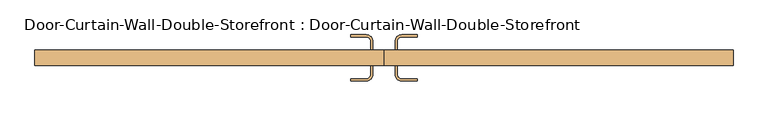
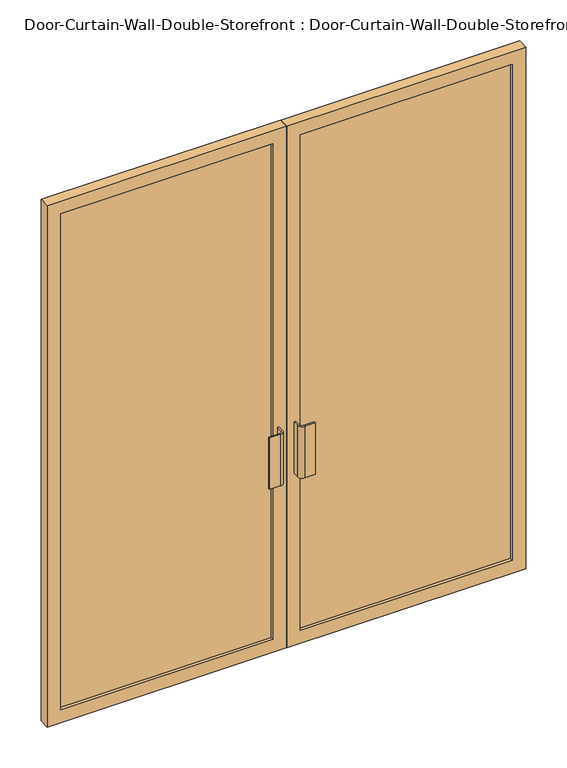
"""IFC4 building model written with IfcOpenShell, lengths in millimetres: door geometry, Door-Curtain-Wall-Double-Storefront : Door-Curtain-Wall-Double-Storefront."""

from ifc_helpers import new_model, si_unit, point, frame, frame_2d, origin, place, context, project, spatial, polyline, circle_curve, trimmed, segment, composite_curve, outline, extrude, source, transform, mapped, element, save


def door_curtain_wall_double_storefront_door_curtain_wall_double_726648f4(model_context):
    return source(origin(), model_context, "Body", "SweptSolid", [
        extrude(outline(polyline([(2311.4, 0.7668501), (0.0, 0.7668501), (0.0, 1003.3), (2311.4, 1003.3), (2311.4, 0.7668501)]), holes=[polyline([(2254.25, 57.9168501), (2254.25, 946.15), (57.15, 946.15), (57.15, 57.9168501), (2254.25, 57.9168501)])]), frame((0.0, 12.7, 0.0), z_axis=(0.0, 1.0, 0.0), x_axis=(0.0, 0.0, 1.0)), (0.0, 0.0, 1.0), 44.45),
        extrude(outline(polyline([(2311.4, -0.8206499), (2311.4, -1003.3), (0.0, -1003.3), (0.0, -0.8206499), (2311.4, -0.8206499)]), holes=[polyline([(2254.25, -946.15), (2254.25, -57.9706499), (57.15, -57.9706499), (57.15, -946.15), (2254.25, -946.15)])]), frame((0.0, 12.7, 0.0), z_axis=(0.0, 1.0, 0.0), x_axis=(0.0, 0.0, 1.0)), (0.0, 0.0, 1.0), 44.45),
        extrude(outline(polyline([(946.15, 25.4), (57.9168501, 25.4), (57.9168501, 44.45), (946.15, 44.45), (946.15, 25.4)])), frame((0.0, 0.0, 57.15), z_axis=(0.0, 0.0, 1.0), x_axis=(1.0, 0.0, 0.0)), (0.0, 0.0, 1.0), 2197.1),
        extrude(outline(polyline([(-57.9706499, 25.4), (-946.15, 25.4), (-946.15, 44.45), (-57.9706499, 44.45), (-57.9706499, 25.4)])), frame((0.0, 0.0, 57.15), z_axis=(0.0, 0.0, 1.0), x_axis=(1.0, 0.0, 0.0)), (0.0, 0.0, 1.0), 2197.1),
        extrude(outline(composite_curve([segment(polyline([(-31.7768999, 82.55), (-31.7768999, 57.15), (-38.1268999, 57.15), (-38.1268999, 82.55)]), True, "CONTINUOUS"), segment(trimmed(circle_curve(frame_2d((-50.8268999, 82.55)), 12.7), [point((-38.1268999, 82.55))], [point((-50.8268999, 95.25))], True, "CARTESIAN"), True, "CONTINUOUS"), segment(polyline([(-50.8268999, 95.25), (-95.2768999, 95.25), (-95.2768999, 101.6), (-50.8268999, 101.6)]), True, "CONTINUOUS"), segment(trimmed(circle_curve(frame_2d((-50.8268999, 82.55)), 19.05), [point((-50.8268999, 101.6))], [point((-31.7768999, 82.55))], False, "CARTESIAN"), True, "CONTINUOUS")], self_intersect=False)), frame((0.0, 0.0, 762.0), z_axis=(0.0, 0.0, 1.0), x_axis=(1.0, 0.0, 0.0)), (0.0, 0.0, 1.0), 228.6),
        extrude(outline(composite_curve([segment(trimmed(circle_curve(frame_2d((50.7731001, 82.55)), 19.05), [point((31.7231001, 82.55))], [point((50.7731001, 101.6))], False, "CARTESIAN"), True, "CONTINUOUS"), segment(polyline([(50.7731001, 101.6), (95.2231001, 101.6), (95.2231001, 95.25), (50.7731001, 95.25)]), True, "CONTINUOUS"), segment(trimmed(circle_curve(frame_2d((50.7731001, 82.55)), 12.7), [point((50.7731001, 95.25))], [point((38.0731001, 82.55))], True, "CARTESIAN"), True, "CONTINUOUS"), segment(polyline([(38.0731001, 82.55), (38.0731001, 57.15), (31.7231001, 57.15), (31.7231001, 82.55)]), True, "CONTINUOUS")], self_intersect=False)), frame((0.0, 0.0, 762.0), z_axis=(0.0, 0.0, 1.0), x_axis=(1.0, 0.0, 0.0)), (0.0, 0.0, 1.0), 228.6),
        extrude(outline(composite_curve([segment(trimmed(circle_curve(frame_2d((-50.8268999, -12.7)), 19.05), [point((-31.7768999, -12.7))], [point((-50.8268999, -31.75))], False, "CARTESIAN"), True, "CONTINUOUS"), segment(polyline([(-50.8268999, -31.75), (-95.2768999, -31.75), (-95.2768999, -25.4), (-50.8268999, -25.4)]), True, "CONTINUOUS"), segment(trimmed(circle_curve(frame_2d((-50.8268999, -12.7)), 12.7), [point((-50.8268999, -25.4))], [point((-38.1268999, -12.7))], True, "CARTESIAN"), True, "CONTINUOUS"), segment(polyline([(-38.1268999, -12.7), (-38.1268999, 12.7), (-31.7768999, 12.7), (-31.7768999, -12.7)]), True, "CONTINUOUS")], self_intersect=False)), frame((0.0, 0.0, 762.0), z_axis=(0.0, 0.0, 1.0), x_axis=(1.0, 0.0, 0.0)), (0.0, 0.0, 1.0), 228.6),
        extrude(outline(composite_curve([segment(polyline([(31.7231001, -12.7), (31.7231001, 12.7), (38.0731001, 12.7), (38.0731001, -12.7)]), True, "CONTINUOUS"), segment(trimmed(circle_curve(frame_2d((50.7731001, -12.7)), 12.7), [point((38.0731001, -12.7))], [point((50.7731001, -25.4))], True, "CARTESIAN"), True, "CONTINUOUS"), segment(polyline([(50.7731001, -25.4), (95.2231001, -25.4), (95.2231001, -31.75), (50.7731001, -31.75)]), True, "CONTINUOUS"), segment(trimmed(circle_curve(frame_2d((50.7731001, -12.7)), 19.05), [point((50.7731001, -31.75))], [point((31.7231001, -12.7))], False, "CARTESIAN"), True, "CONTINUOUS")], self_intersect=False)), frame((0.0, 0.0, 762.0), z_axis=(0.0, 0.0, 1.0), x_axis=(1.0, 0.0, 0.0)), (0.0, 0.0, 1.0), 228.6),
    ])


if __name__ == "__main__":
    model = new_model("IFC4")
    model_context = context("Model", 3, world=origin())
    ifc_project = project(units=[si_unit("LENGTHUNIT", "METRE", prefix="MILLI")], contexts=[model_context])
    site = spatial("IfcSite", under=ifc_project)
    building = spatial("IfcBuilding", under=site)
    placement = place(None, origin())
    door_curtain_wall_double_storefront_door_curtain_wall_double_shape = door_curtain_wall_double_storefront_door_curtain_wall_double_726648f4(model_context)
    element("IfcDoor", 1, ObjectType="Door-Curtain-Wall-Double-Storefront : Door-Curtain-Wall-Double-Storefront", at=placement, inside=building, context=model_context, shape_type="MappedRepresentation", body=[
        mapped(door_curtain_wall_double_storefront_door_curtain_wall_double_shape, transform((0.0, 0.0, 0.0), x_axis=(1.0, 0.0, 0.0), y_axis=(0.0, 1.0, 0.0), z_axis=(0.0, 0.0, 1.0))),
    ])
    save(model, "model.ifc")

# Revit data of these elements
# Type "Door-Curtain-Wall-Double-Storefront : Door-Curtain-Wall-Double-Storefront"
#   Type Mark = "9"
#   Construction Type Id = "opn-d46"
#   Assembly Code = "B2030100"
#   Analytic Construction = "Metal frame, double glass door"
#   Width [instance default] = 6' - 0"
#   Thermal Resistance (R) = 1.3794 (h·ft²·°F)/BTU
#   Swing Angle [instance default] = 90.00°
#   Panel Width [instance default] = 3' - 0"
#   Offset = 0' - 2 1/4"
#   Heat Transfer Coefficient (U) = 0.7250 BTU/(h·ft²·°F)
#   Define Thermal Properties by = 1
#   Function = 1
#   Frame Material = Aluminum
#   Door Handle Material = Aluminum
#   Glazing = Glass
#   Visual Light Transmittance = 0
#   Solar Heat Gain Coefficient = 0
# Element 1 (IfcDoor, "Door-Curtain-Wall-Double-Storefront : Door-Curtain-Wall-Double-Storefront")
#   Width = 6' - 7"
#   Panel Width = 3' - 3 1/2"
#   Materials on its faces: "Aluminum", "Glass"
# Materials
#   "Aluminum": class "Metal", colour RGB 247 247 247, transparency 0, Description = "Aluminum 6061", Cost = 0
#   "Glass": class "Glass", colour RGB 0 128 192, transparency 0.75, Description = "Soda Lime Glass", Cost = 0
